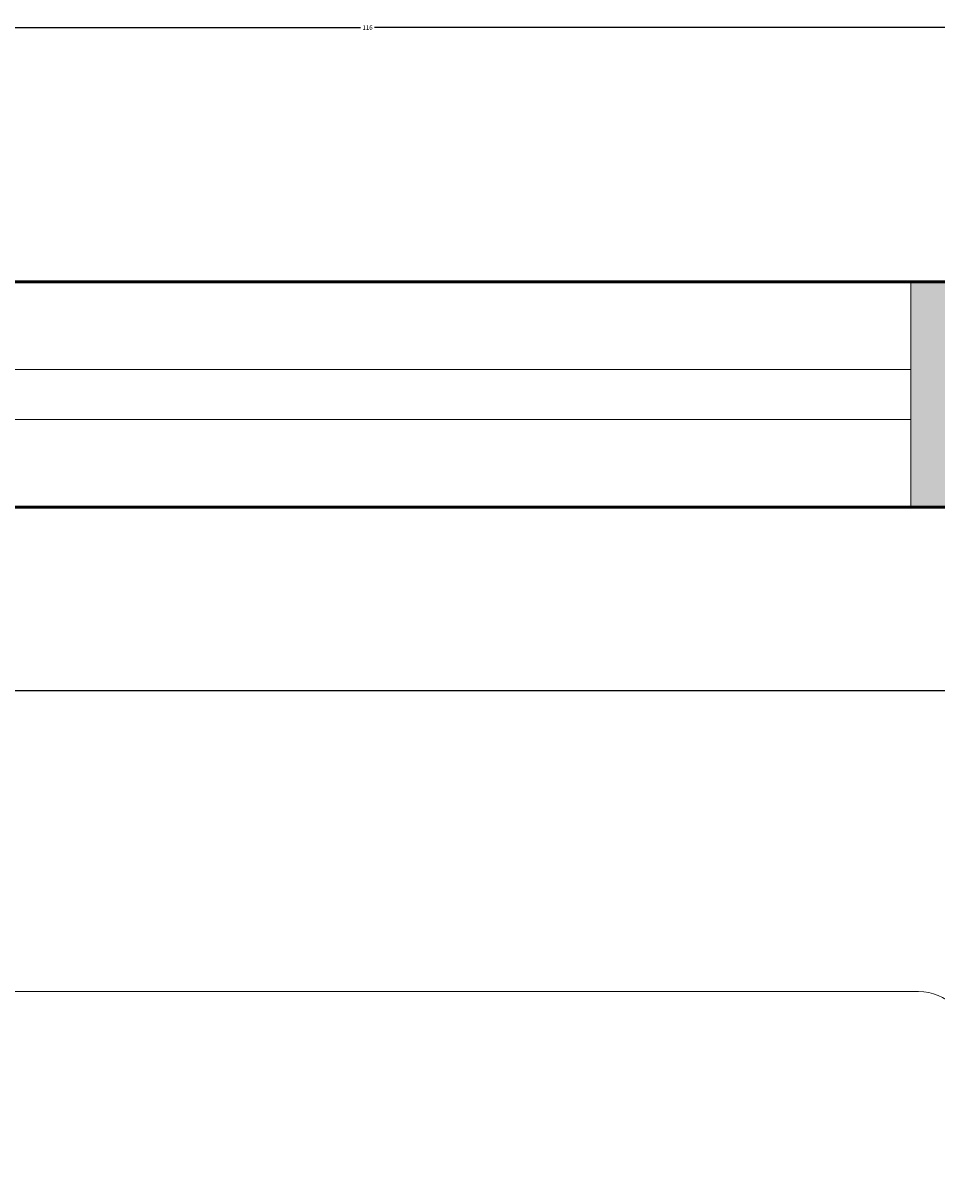
# Model space of a CAD drawing. Units: inches. Extents: x 2307 to 2544, y 2171 to 2540.
# Tile 26 of 52: x 2380 to 2416, y 2485 to 2531. Entities that reach past the tile are written whole.
import ezdxf

# ---------------------------------------------------------------- set-up
doc = ezdxf.new("R2010")
doc.units = ezdxf.units.IN
for name, color, linetype, lineweight in [('A-ANNO-DIMS', 2, 'Continuous', 18), ('A-FURN', 8, 'Continuous', 18), ('A-GLAZ', 4, 'Continuous', 18), ('A-WALL', 7, 'Continuous', 50)]:
    doc.layers.add(name, color=color, linetype=linetype, lineweight=lineweight)
doc.layers.add('A-WALL-PATT', color=18, linetype='Continuous', lineweight=13, true_color=0x000000)
doc.styles.get("Standard").update_dxf_attribs({"font": 'arial.ttf'})
doc.dimstyles.get("Standard").update_dxf_attribs({"dimtxt": 0.18, "dimasz": 0.18, "dimexe": 0.18, "dimexo": 0.0625, "dimgap": 0.09, "dimtad": 0, "dimtih": 1, "dimtoh": 1, "dimdec": 4, "dimzin": 0, "dimdsep": 46, "dimtxsty": 'Standard', "dimcen": 0.09, "dimadec": 0, "dimazin": 0, "dimtfac": 1, "dimtdec": 4, "dimtofl": 0, "dimtmove": 0, "dimatfit": 3, "dimfxl": 1, "dimtolj": 1, "dimtzin": 0, "dimarcsym": 0})

# ---------------------------------------------------------------- blocks, each defined once
blk = doc.blocks.new('Bed - Queen')
blk.add_line((59.99999, -2), (59.99999, -78.00003))
blk.add_arc((57.99999, -78.00003), 2, 270, 0)
blk = doc.blocks.new('WIN-48IN')
for p, q in [((0, 5.5), (48, 5.5)), ((0, 3.5), (48, 3.5))]:
    blk.add_line(p, q)
for points in [[(0, 0), (0, 9)], [(48, 9), (48, 0)]]:
    blk.add_lwpolyline(points)
blk = doc.blocks.new('*D26')
at = {"layer": 'A-ANNO-DIMS', "color": 0, "lineweight": -2, "transparency": 16777216}
for p, q in [((2337.708, 2492.237), (2337.708, 2504.354)), ((2417.708, 2492.237), (2417.708, 2504.354)), ((2337.888, 2504.174), (2376.714, 2504.174)), ((2417.528, 2504.174), (2378.702, 2504.174))]:
    blk.add_line(p, q, dxfattribs=at)
at = {"layer": 'A-ANNO-DIMS', "color": 0, "transparency": 16777216}
for points in [[(2337.888, 2504.204), (2337.888, 2504.144), (2337.708, 2504.174)], [(2417.528, 2504.204), (2417.528, 2504.144), (2417.708, 2504.174)]]:
    blk.add_solid(points, dxfattribs=at)
at = {"layer": 'Defpoints', "color": 0, "transparency": 16777216}
for p in [(2337.708, 2504.174), (2337.708, 2492.174), (2417.708, 2492.174)]:
    blk.add_point(p, dxfattribs=at)
at = {"layer": 'A-ANNO-DIMS', "color": 0, "transparency": 16777216, "insert": (2377.708, 2504.174), "char_height": 0.18, "attachment_point": 5}
blk.add_mtext('\\A1;QUEEN BED 80', dxfattribs=at)
blk = doc.blocks.new('*D45')
at = {"layer": 'A-ANNO-DIMS', "color": 0, "lineweight": -2, "transparency": 16777216}
for p, q in [((2335.696, 2511.572), (2335.696, 2530.84)), ((2335.876, 2530.66), (2393.416, 2530.66)), ((2451.516, 2530.66), (2393.976, 2530.66)), ((2451.696, 2511.572), (2451.696, 2530.84))]:
    blk.add_line(p, q, dxfattribs=at)
at = {"layer": 'A-ANNO-DIMS', "color": 0, "transparency": 16777216}
for points in [[(2335.876, 2530.69), (2335.876, 2530.63), (2335.696, 2530.66)], [(2451.516, 2530.69), (2451.516, 2530.63), (2451.696, 2530.66)]]:
    blk.add_solid(points, dxfattribs=at)
at = {"layer": 'Defpoints', "color": 0, "transparency": 16777216}
for p in [(2451.696, 2530.66), (2335.696, 2511.51), (2451.696, 2511.51)]:
    blk.add_point(p, dxfattribs=at)
at = {"layer": 'A-ANNO-DIMS', "color": 0, "transparency": 16777216, "insert": (2393.696, 2530.66), "char_height": 0.18, "attachment_point": 5}
blk.add_mtext('\\A1;116', dxfattribs=at)
blk = doc.blocks.new('*D48')
at = {"layer": 'A-ANNO-DIMS', "color": 0, "lineweight": -2, "transparency": 16777216}
for p, q in [((2455.633, 2511.51), (2307.366, 2511.51)), ((2307.546, 2511.33), (2307.546, 2475.69)), ((2307.546, 2439.69), (2307.546, 2475.329)), ((2455.633, 2439.51), (2307.366, 2439.51))]:
    blk.add_line(p, q, dxfattribs=at)
at = {"layer": 'A-ANNO-DIMS', "color": 0, "transparency": 16777216}
for points in [[(2307.516, 2511.33), (2307.576, 2511.33), (2307.546, 2511.51)], [(2307.516, 2439.69), (2307.576, 2439.69), (2307.546, 2439.51)]]:
    blk.add_solid(points, dxfattribs=at)
at = {"layer": 'Defpoints', "color": 0, "transparency": 16777216}
for p in [(2307.546, 2511.51), (2455.696, 2511.51), (2455.696, 2439.51)]:
    blk.add_point(p, dxfattribs=at)
at = {"layer": 'A-ANNO-DIMS', "color": 0, "transparency": 16777216, "insert": (2307.546, 2475.51), "char_height": 0.18, "attachment_point": 5}
blk.add_mtext('\\A1;72', dxfattribs=at)

msp = doc.modelspace()

# ---------------------------------------------------------------- hatches: boundary and pattern name
at = {"layer": 'A-WALL-PATT'}
h = msp.add_hatch(color=256, dxfattribs=at)
h.dxf.hatch_style = 1
h.paths.add_polyline_path([(2433.6935, 2199.5096), (2415.6423, 2199.5096), (2415.6423, 2190.5096), (2433.7832, 2190.5096)], flags=17)
h.paths.add_polyline_path([(2367.6423, 2199.5096), (2335.6958, 2199.5096), (2335.6958, 2307.3983), (2326.6958, 2307.3983), (2326.6958, 2190.5096), (2367.6423, 2190.5096)])
h.paths.add_polyline_path([(2524.6958, 2520.5096), (2496.7832, 2520.5096), (2496.7832, 2515.5149), (2472.7832, 2515.5149), (2472.7832, 2520.5096), (2415.4028, 2520.5096), (2415.4028, 2511.5096), (2451.6958, 2511.5096), (2451.6958, 2439.5096), (2451.6958, 2391.5096), (2445.6958, 2391.5096), (2445.6958, 2387.5096), (2455.6958, 2387.5096), (2455.6958, 2435.5096), (2461.6958, 2435.5096), (2461.6958, 2439.5096), (2455.6958, 2439.5096), (2455.6958, 2511.5096), (2515.6958, 2511.5096), (2515.6958, 2439.5096), (2491.6958, 2439.5096), (2491.6958, 2435.5096), (2515.6958, 2435.5096), (2515.6958, 2319.5096), (2451.6958, 2319.5096), (2451.6958, 2281.5096), (2481.6958, 2281.5096), (2481.6958, 2225.5096), (2485.6958, 2225.5096), (2485.6958, 2285.5096), (2455.6958, 2285.5096), (2455.6958, 2315.5096), (2515.6958, 2315.5096), (2515.6958, 2199.5096), (2469.6952, 2199.5096), (2469.785, 2190.5096), (2524.6958, 2190.5096)])

# ---------------------------------------------------------------- linework, layer by layer
at = {"layer": 'A-WALL'}
msp.add_line((2335.6958, 2511.5096), (2451.6958, 2511.5096), dxfattribs=at)
msp.add_lwpolyline([(2433.7832, 2190.5096), (2326.6958, 2190.5096), (2326.6958, 2520.5096), (2524.6958, 2520.5096), (2524.6958, 2190.5096), (2469.785, 2190.5096)], dxfattribs=at)

# ---------------------------------------------------------------- block references
at = {"layer": 'A-FURN', "rotation": 90}
msp.add_blockref('Bed - Queen', (2337.7083, 2432.1742), dxfattribs=at)
at = {"layer": 'A-GLAZ', "rotation": 180}
msp.add_blockref('WIN-48IN', (2415.4031, 2520.5091), dxfattribs=at)

# ---------------------------------------------------------------- dimensions: what is measured, and where the dimension line sits
at = {"layer": 'A-ANNO-DIMS'}
dim = msp.add_linear_dim(base=(2451.6958, 2530.6596), p1=(2335.6958, 2511.5096), p2=(2451.6958, 2511.5096), dimstyle='Standard', override={"dimdec": 0, "dimlfac": 1, "dimrnd": 0, "dimzin": 0, "dimdsep": 46, "dimlunit": 2}, dxfattribs=at)
dim.commit()
dim.dimension.update_dxf_attribs({"geometry": '*D45', "text_midpoint": (2393.6958, 2530.6596)})
dim = msp.add_linear_dim(base=(2307.5458, 2511.5096), p1=(2455.6958, 2439.5096), p2=(2455.6958, 2511.5096), angle=90, dimstyle='Standard', override={"dimdec": 0, "dimlfac": 1, "dimrnd": 0, "dimzin": 0, "dimdsep": 46, "dimlunit": 2}, dxfattribs=at)
dim.commit()
dim.dimension.update_dxf_attribs({"geometry": '*D48', "text_midpoint": (2307.5458, 2475.5096)})
dim = msp.add_linear_dim(base=(2337.7083, 2504.1742), p1=(2417.7084, 2492.1742), p2=(2337.7083, 2492.1742), angle=180, text='QUEEN BED <>', dimstyle='Standard', override={"dimdec": 0, "dimlfac": 1, "dimrnd": 0, "dimzin": 0, "dimdsep": 46, "dimlunit": 2}, dxfattribs=at)
dim.commit()
dim.dimension.update_dxf_attribs({"geometry": '*D26', "text_midpoint": (2377.7083, 2504.1742)})

doc.saveas('drawing.dxf')
